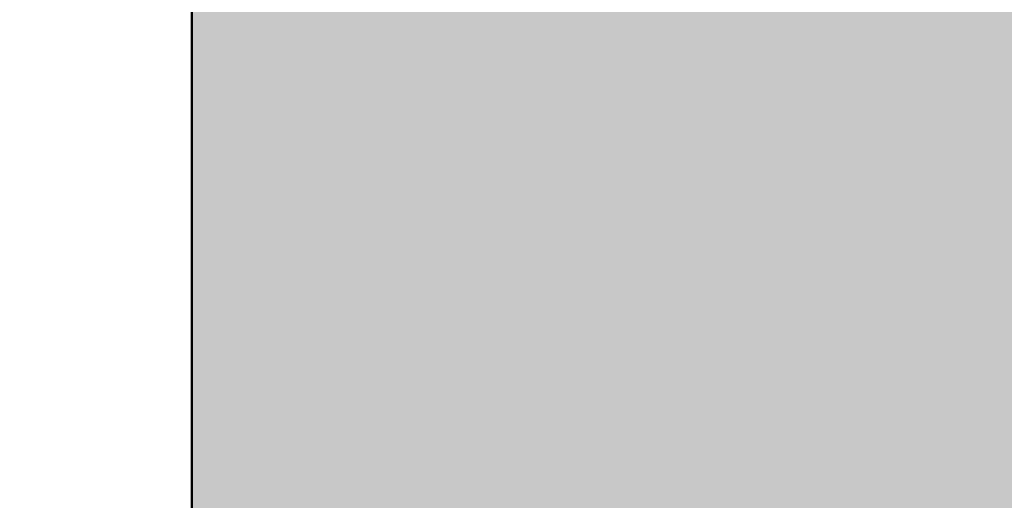
# Model space of a CAD drawing. Units: millimetres. Extents: x 0 to 2267, y 0 to 1823.
# Tile 29 of 256: x 1590 to 1611, y 1216 to 1226. Entities that reach past the tile are written whole.
import ezdxf

# ---------------------------------------------------------------- set-up
doc = ezdxf.new("R2010")
doc.units = ezdxf.units.MM
doc.header["$MEASUREMENT"] = 0
doc.layers.add('M-HATC', color=252, linetype='Continuous', lineweight=18)
doc.layers.add('M-OUTL', color=7, linetype='Continuous', lineweight=50)

msp = doc.modelspace()

# ---------------------------------------------------------------- hatches: boundary and pattern name
at = {"layer": 'M-HATC'}
h = msp.add_hatch(color=256, dxfattribs=at)
h.dxf.hatch_style = 1
h.paths.add_polyline_path([(2055.771, 1603.062), (1381.087, 1603.062), (1381.087, 1598.062), (2055.771, 1598.062)])
h.paths.add_polyline_path([(2055.771, 1598.062), (1381.087, 1598.062), (1381.087, 1593.062), (2055.771, 1593.062)])
h.paths.add_polyline_path([(2051.307, 1536.761), (1385.55, 1536.761), (1385.55, 1526.761), (1387.55, 1526.761), (1388.537, 1525.053), (1385.332, 1521.233), (1385.332, 1521.223), (2050.254, 1522.749), (2048.321, 1525.053), (2049.307, 1526.761), (2051.307, 1526.761)])
edge = h.paths.add_edge_path()
edge.add_arc((1847.535, 1379.149), 135, 222.60306, 222.89085, ccw=False)
edge.add_line((1748.166, 1287.766), (1683.092, 1287.766))
edge.add_arc((1583.724, 1379.149), 135, 317.10915, 317.39694, ccw=False)
edge.add_arc((1678.969, 1290.671), 5, 222.8909, 317.1091, ccw=False)
edge.add_arc((1774.213, 1379.149), 135, 222.60306, 222.89085, ccw=False)
edge.add_line((1674.845, 1287.766), (1609.771, 1287.766))
edge.add_arc((1510.403, 1379.149), 135, 317.10915, 317.39694, ccw=False)
edge.add_arc((1605.647, 1290.671), 5, 222.8909, 317.1091, ccw=False)
edge.add_arc((1700.892, 1379.149), 135, 222.60306, 222.89085, ccw=False)
edge.add_line((1601.524, 1287.766), (1536.45, 1287.766))
edge.add_arc((1437.081, 1379.149), 135, 317.10915, 317.39694, ccw=False)
edge.add_arc((1532.326, 1290.671), 5, 222.8909, 317.1091, ccw=False)
edge.add_arc((1627.571, 1379.149), 135, 222.60306, 222.89085, ccw=False)
edge.add_line((1528.203, 1287.766), (1505.929, 1287.766))
edge.add_spline(control_points=[(1505.929, 1287.766), (1504.262, 1287.766), (1504.262, 1282.766), (1505.929, 1282.766)], knot_values=[0, 0, 0, 0, 5, 5, 5, 5], degree=3, periodic=0)
edge.add_line((1505.929, 1282.766), (1930.929, 1282.766))
edge.add_spline(control_points=[(1930.929, 1282.766), (1932.596, 1282.766), (1932.596, 1287.766), (1930.929, 1287.766)], knot_values=[0, 0, 0, 0, 5, 5, 5, 5], degree=3, periodic=0)
edge.add_line((1930.929, 1287.766), (1903.056, 1287.766))
edge.add_arc((1803.688, 1379.149), 135, 317.10915, 317.39694, ccw=False)
edge.add_arc((1898.932, 1290.671), 5, 222.8909, 317.1091, ccw=False)
edge.add_arc((1994.177, 1379.149), 135, 222.60306, 222.89085, ccw=False)
edge.add_line((1894.809, 1287.766), (1829.735, 1287.766))
edge.add_arc((1730.366, 1379.149), 135, 317.10915, 317.39694, ccw=False)
edge.add_arc((1825.611, 1290.671), 5, 222.8909, 317.1091, ccw=False)
edge.add_arc((1920.856, 1379.149), 135, 222.60306, 222.89085, ccw=False)
edge.add_line((1821.487, 1287.766), (1756.413, 1287.766))
edge.add_arc((1657.045, 1379.149), 135, 317.10915, 317.39694, ccw=False)
edge.add_arc((1752.29, 1290.671), 5, 222.8909, 317.1091, ccw=False)
edge = h.paths.add_edge_path()
edge.add_spline(control_points=[(1843.429, 1227.247), (1845.096, 1227.247), (1845.096, 1232.247), (1843.429, 1232.247)], knot_values=[0, 0, 0, 0, 5, 5, 5, 5], degree=3, periodic=0)
edge.add_line((1843.429, 1232.247), (1593.429, 1232.247))
edge.add_spline(control_points=[(1593.429, 1232.247), (1591.762, 1232.247), (1591.762, 1227.247), (1593.429, 1227.247)], knot_values=[0, 0, 0, 0, 5, 5, 5, 5], degree=3, periodic=0)
edge.add_line((1593.429, 1227.247), (1843.429, 1227.247))
h.paths.add_polyline_path([(1905.929, 1127.417), (1530.929, 1127.417, 0.414214), (1520.929, 1117.417), (1530.929, 1117.417), (1915.929, 1117.417, 0.414214)])
edge = h.paths.add_edge_path()
edge.add_arc((1397.086, 1498.408), 12.73, 90.7821, 190.8787, ccw=False)
edge.add_line((1396.912, 1511.136), (1428.01, 1511.349))
edge.add_line((1428.01, 1511.349), (1433.01, 1511.349))
edge.add_line((1433.01, 1511.349), (1434.439, 1511.349))
edge.add_arc((1419.474, 1498.08), 20, 41.561, 74.0821)
edge.add_line((1424.959, 1517.314), (1399.935, 1517.256))
edge.add_spline(control_points=[(1399.931, 1517.256), (1399.884, 1517.213), (1399.833, 1517.169), (1399.777, 1517.124)], knot_values=[11.567499, 11.567499, 11.567499, 11.567499, 11.814249, 11.814249, 11.814249, 11.814249], degree=3, periodic=0)
edge.add_spline(control_points=[(1399.633, 1517.01), (1399.583, 1516.972), (1399.531, 1516.934), (1399.476, 1516.895)], knot_values=[11.167718, 11.167718, 11.167718, 11.167718, 11.365188, 11.365188, 11.365188, 11.365188], degree=3, periodic=0)
edge.add_spline(control_points=[(1399.34, 1516.8), (1399.151, 1516.672), (1398.938, 1516.538), (1398.704, 1516.399)], knot_values=[10.376405, 10.376405, 10.376405, 10.376405, 11.00994, 11.00994, 11.00994, 11.00994], degree=3, periodic=0)
edge.add_spline(control_points=[(1398.657, 1516.372), (1398.579, 1516.326), (1398.498, 1516.28), (1398.415, 1516.233)], knot_values=[10.125175, 10.125175, 10.125175, 10.125175, 10.334406, 10.334406, 10.334406, 10.334406], degree=3, periodic=0)
edge.add_spline(control_points=[(1398.264, 1516.149), (1398.196, 1516.111), (1398.126, 1516.073), (1398.055, 1516.035)], knot_values=[9.832246, 9.832246, 9.832246, 9.832246, 9.999658, 9.999658, 9.999658, 9.999658], degree=3, periodic=0)
edge.add_spline(control_points=[(1397.999, 1516.005), (1397.731, 1515.862), (1397.446, 1515.717), (1397.147, 1515.571)], knot_values=[9.161808, 9.161808, 9.161808, 9.161808, 9.787769, 9.787769, 9.787769, 9.787769], degree=3, periodic=0)
edge.add_spline(control_points=[(1397.147, 1515.571), (1396.842, 1515.423), (1396.522, 1515.274), (1396.191, 1515.126)], knot_values=[8.524455, 8.524455, 8.524455, 8.524455, 9.161808, 9.161808, 9.161808, 9.161808], degree=3, periodic=0)
edge.add_spline(control_points=[(1396.078, 1515.076), (1395.985, 1515.035), (1395.892, 1514.994), (1395.798, 1514.953)], knot_values=[8.275193, 8.275193, 8.275193, 8.275193, 8.451726, 8.451726, 8.451726, 8.451726], degree=3, periodic=0)
edge.add_spline(control_points=[(1395.602, 1514.869), (1395.5, 1514.826), (1395.397, 1514.782), (1395.293, 1514.739)], knot_values=[7.962917, 7.962917, 7.962917, 7.962917, 8.152764, 8.152764, 8.152764, 8.152764], degree=3, periodic=0)
edge.add_spline(control_points=[(1395.212, 1514.706), (1394.828, 1514.547), (1394.435, 1514.393), (1394.036, 1514.244)], knot_values=[7.21254, 7.21254, 7.21254, 7.21254, 7.913148, 7.913148, 7.913148, 7.913148], degree=3, periodic=0)
edge.add_spline(control_points=[(1394.036, 1514.244), (1393.708, 1514.121), (1393.375, 1514.003), (1393.043, 1513.889)], knot_values=[6.633733, 6.633733, 6.633733, 6.633733, 7.21254, 7.21254, 7.21254, 7.21254], degree=3, periodic=0)
edge.add_spline(control_points=[(1392.821, 1513.815), (1392.72, 1513.781), (1392.618, 1513.748), (1392.517, 1513.715)], knot_values=[6.328796, 6.328796, 6.328796, 6.328796, 6.505493, 6.505493, 6.505493, 6.505493], degree=3, periodic=0)
edge.add_spline(control_points=[(1392.517, 1513.715), (1392.319, 1513.652), (1392.121, 1513.59), (1391.924, 1513.531)], knot_values=[5.984605, 5.984605, 5.984605, 5.984605, 6.328796, 6.328796, 6.328796, 6.328796], degree=3, periodic=0)
edge.add_spline(control_points=[(1391.792, 1513.491), (1391.312, 1513.35), (1390.838, 1513.224), (1390.378, 1513.117)], knot_values=[5.066697, 5.066697, 5.066697, 5.066697, 5.907055, 5.907055, 5.907055, 5.907055], degree=3, periodic=0)
edge.add_spline(control_points=[(1390.378, 1513.117), (1390.18, 1513.071), (1389.984, 1513.028), (1389.791, 1512.99)], knot_values=[4.70367, 4.70367, 4.70367, 4.70367, 5.066695, 5.066695, 5.066695, 5.066695], degree=3, periodic=0)
edge.add_spline(control_points=[(1389.422, 1512.92), (1389.246, 1512.889), (1389.073, 1512.862), (1388.904, 1512.838)], knot_values=[4.130571, 4.130571, 4.130571, 4.130571, 4.469816, 4.469816, 4.469816, 4.469816], degree=3, periodic=0)
edge.add_spline(control_points=[(1388.904, 1512.838), (1388.591, 1512.795), (1388.291, 1512.764), (1388.007, 1512.749)], knot_values=[3.504031, 3.504031, 3.504031, 3.504031, 4.130571, 4.130571, 4.130571, 4.130571], degree=3, periodic=0)
edge.add_spline(control_points=[(1387.936, 1512.746), (1387.854, 1512.742), (1387.773, 1512.74), (1387.694, 1512.739)], knot_values=[3.268866, 3.268866, 3.268866, 3.268866, 3.451164, 3.451164, 3.451164, 3.451164], degree=3, periodic=0)
edge.add_spline(control_points=[(1387.335, 1512.744), (1387.208, 1512.75), (1387.085, 1512.76), (1386.967, 1512.774)], knot_values=[2.670686, 2.670686, 2.670686, 2.670686, 2.984, 2.984, 2.984, 2.984], degree=3, periodic=0)
edge.add_spline(control_points=[(1386.833, 1512.792), (1386.821, 1512.794), (1386.809, 1512.796), (1386.797, 1512.798)], knot_values=[2.516981, 2.516981, 2.516981, 2.516981, 2.549528, 2.549528, 2.549528, 2.549528], degree=3, periodic=0)
edge.add_spline(control_points=[(1386.453, 1512.873), (1386.426, 1512.881), (1386.399, 1512.889), (1386.373, 1512.897)], knot_values=[2.095869, 2.095869, 2.095869, 2.095869, 2.17941, 2.17941, 2.17941, 2.17941], degree=3, periodic=0)
edge.add_spline(control_points=[(1386.069, 1513.019), (1386.063, 1513.022), (1386.058, 1513.025), (1386.052, 1513.028)], knot_values=[1.72453, 1.72453, 1.72453, 1.72453, 1.745933, 1.745933, 1.745933, 1.745933], degree=3, periodic=0)
edge.add_arc((1399.474, 1498.08), 20, 131.8243, 180)
edge.add_arc((1630.334, 1505.548), 250.971, 181.70518, 236.42798)
edge.add_arc((1605.34, 1483.304), 218.782, 238.66083, 243.34961)
edge.add_arc((1647.091, 1510.359), 262.899, 183.12984, 237.85344, ccw=False)
h.paths.add_polyline_path([(1406.537, 1391.964, 0.149382), (1491.551, 1296.442, -0.129517)], flags=17)
edge = h.paths.add_edge_path()
edge.add_arc((2037.384, 1498.08), 20, 0, 48.2659)
edge.add_spline(control_points=[(2050.697, 1513.005), (2050.651, 1512.985), (2050.603, 1512.966), (2050.554, 1512.948)], knot_values=[1.835652, 1.835652, 1.835652, 1.835652, 2.000781, 2.000781, 2.000781, 2.000781], degree=3, periodic=0)
edge.add_spline(control_points=[(2050.462, 1512.917), (2050.479, 1512.922), (2050.496, 1512.928), (2050.513, 1512.934)], knot_values=[2.045477, 2.045477, 2.045477, 2.045477, 2.101389, 2.101389, 2.101389, 2.101389], degree=3, periodic=0)
edge.add_spline(control_points=[(2050.129, 1512.834), (2050.198, 1512.847), (2050.266, 1512.862), (2050.331, 1512.879)], knot_values=[2.237629, 2.237629, 2.237629, 2.237629, 2.435841, 2.435841, 2.435841, 2.435841], degree=3, periodic=0)
edge.add_spline(control_points=[(2050.095, 1512.828), (2050.106, 1512.83), (2050.118, 1512.832), (2050.129, 1512.834)], knot_values=[2.435841, 2.435841, 2.435841, 2.435841, 2.468321, 2.468321, 2.468321, 2.468321], degree=3, periodic=0)
edge.add_spline(control_points=[(2049.784, 1512.785), (2049.855, 1512.792), (2049.924, 1512.801), (2049.992, 1512.811)], knot_values=[2.563852, 2.563852, 2.563852, 2.563852, 2.748541, 2.748541, 2.748541, 2.748541], degree=3, periodic=0)
edge.add_spline(control_points=[(2049.405, 1512.762), (2049.536, 1512.765), (2049.663, 1512.773), (2049.784, 1512.785)], knot_values=[2.748541, 2.748541, 2.748541, 2.748541, 3.064882, 3.064882, 3.064882, 3.064882], degree=3, periodic=0)
edge.add_spline(control_points=[(2049.17, 1512.76), (2049.234, 1512.759), (2049.297, 1512.759), (2049.358, 1512.761)], knot_values=[3.102309, 3.102309, 3.102309, 3.102309, 3.2503, 3.2503, 3.2503, 3.2503], degree=3, periodic=0)
edge.add_spline(control_points=[(2048.857, 1512.769), (2048.964, 1512.764), (2049.068, 1512.761), (2049.17, 1512.76)], knot_values=[3.2503, 3.2503, 3.2503, 3.2503, 3.486069, 3.486069, 3.486069, 3.486069], degree=3, periodic=0)
edge.add_spline(control_points=[(2048.692, 1512.779), (2048.373, 1512.801), (2048.035, 1512.841), (2047.682, 1512.897)], knot_values=[3.606429, 3.606429, 3.606429, 3.606429, 4.2989, 4.2989, 4.2989, 4.2989], degree=3, periodic=0)
edge.add_spline(control_points=[(2047.682, 1512.897), (2047.546, 1512.919), (2047.408, 1512.942), (2047.268, 1512.969)], knot_values=[4.2989, 4.2989, 4.2989, 4.2989, 4.565769, 4.565769, 4.565769, 4.565769], degree=3, periodic=0)
edge.add_spline(control_points=[(2047.268, 1512.969), (2047.145, 1512.991), (2047.021, 1513.016), (2046.895, 1513.042)], knot_values=[4.565769, 4.565769, 4.565769, 4.565769, 4.799971, 4.799971, 4.799971, 4.799971], degree=3, periodic=0)
edge.add_spline(control_points=[(2046.895, 1513.042), (2046.529, 1513.119), (2046.151, 1513.209), (2045.768, 1513.311)], knot_values=[4.799971, 4.799971, 4.799971, 4.799971, 5.483718, 5.483718, 5.483718, 5.483718], degree=3, periodic=0)
edge.add_spline(control_points=[(2045.768, 1513.311), (2045.372, 1513.415), (2044.97, 1513.532), (2044.566, 1513.659)], knot_values=[5.483718, 5.483718, 5.483718, 5.483718, 6.187866, 6.187866, 6.187866, 6.187866], degree=3, periodic=0)
edge.add_spline(control_points=[(2044.566, 1513.659), (2044.415, 1513.706), (2044.263, 1513.755), (2044.112, 1513.805)], knot_values=[6.187866, 6.187866, 6.187866, 6.187866, 6.451551, 6.451551, 6.451551, 6.451551], degree=3, periodic=0)
edge.add_spline(control_points=[(2044.112, 1513.805), (2043.997, 1513.843), (2043.882, 1513.881), (2043.767, 1513.92)], knot_values=[6.451551, 6.451551, 6.451551, 6.451551, 6.651434, 6.651434, 6.651434, 6.651434], degree=3, periodic=0)
edge.add_spline(control_points=[(2043.767, 1513.92), (2043.372, 1514.055), (2042.977, 1514.198), (2042.589, 1514.346)], knot_values=[6.651434, 6.651434, 6.651434, 6.651434, 7.338879, 7.338879, 7.338879, 7.338879], degree=3, periodic=0)
edge.add_spline(control_points=[(2042.589, 1514.346), (2042.164, 1514.507), (2041.746, 1514.675), (2041.341, 1514.846)], knot_values=[7.338879, 7.338879, 7.338879, 7.338879, 8.089209, 8.089209, 8.089209, 8.089209], degree=3, periodic=0)
edge.add_spline(control_points=[(2041.341, 1514.846), (2041.103, 1514.946), (2040.869, 1515.048), (2040.64, 1515.15)], knot_values=[8.089209, 8.089209, 8.089209, 8.089209, 8.529587, 8.529587, 8.529587, 8.529587], degree=3, periodic=0)
edge.add_spline(control_points=[(2040.51, 1515.209), (2040.082, 1515.402), (2039.675, 1515.597), (2039.295, 1515.789)], knot_values=[8.613818, 8.613818, 8.613818, 8.613818, 9.44571, 9.44571, 9.44571, 9.44571], degree=3, periodic=0)
edge.add_spline(control_points=[(2039.295, 1515.789), (2039.062, 1515.907), (2038.839, 1516.025), (2038.629, 1516.14)], knot_values=[9.44571, 9.44571, 9.44571, 9.44571, 9.956404, 9.956404, 9.956404, 9.956404], degree=3, periodic=0)
edge.add_spline(control_points=[(2038.629, 1516.14), (2038.519, 1516.2), (2038.412, 1516.26), (2038.309, 1516.319)], knot_values=[9.956404, 9.956404, 9.956404, 9.956404, 10.223542, 10.223542, 10.223542, 10.223542], degree=3, periodic=0)
edge.add_spline(control_points=[(2038.309, 1516.319), (2038.214, 1516.374), (2038.122, 1516.428), (2038.033, 1516.481)], knot_values=[10.223542, 10.223542, 10.223542, 10.223542, 10.47051, 10.47051, 10.47051, 10.47051], degree=3, periodic=0)
edge.add_spline(control_points=[(2038.033, 1516.481), (2037.786, 1516.63), (2037.564, 1516.773), (2037.372, 1516.909)], knot_values=[10.47051, 10.47051, 10.47051, 10.47051, 11.15767, 11.15767, 11.15767, 11.15767], degree=3, periodic=0)
edge.add_spline(control_points=[(2037.372, 1516.909), (2037.279, 1516.975), (2037.193, 1517.04), (2037.114, 1517.102)], knot_values=[11.15767, 11.15767, 11.15767, 11.15767, 11.49227, 11.49227, 11.49227, 11.49227], degree=3, periodic=0)
edge.add_spline(control_points=[(2036.856, 1517.326), (2036.915, 1517.269), (2036.981, 1517.21), (2037.056, 1517.149)], knot_values=[11.577341, 11.577341, 11.577341, 11.577341, 11.91035, 11.91035, 11.91035, 11.91035], degree=3, periodic=0)
edge.add_spline(control_points=[(2036.807, 1517.375), (2036.823, 1517.359), (2036.839, 1517.342), (2036.856, 1517.326)], knot_values=[11.91035, 11.91035, 11.91035, 11.91035, 12.007402, 12.007402, 12.007402, 12.007402], degree=3, periodic=0)
edge.add_spline(control_points=[(2036.702, 1517.494), (2036.71, 1517.483), (2036.72, 1517.472), (2036.729, 1517.461)], knot_values=[12.184155, 12.184155, 12.184155, 12.184155, 12.255409, 12.255409, 12.255409, 12.255409], degree=3, periodic=0)
edge.add_spline(control_points=[(2036.616, 1517.621), (2036.62, 1517.613), (2036.624, 1517.606), (2036.629, 1517.598)], knot_values=[12.487913, 12.487913, 12.487913, 12.487913, 12.541035, 12.541035, 12.541035, 12.541035], degree=3, periodic=0)
edge.add_spline(control_points=[(2036.563, 1517.786), (2036.564, 1517.779), (2036.564, 1517.773), (2036.565, 1517.766)], knot_values=[12.911761, 12.911761, 12.911761, 12.911761, 12.968286, 12.968286, 12.968286, 12.968286], degree=3, periodic=0)
edge.add_spline(control_points=[(2036.617, 1517.93), (2036.612, 1517.926), (2036.609, 1517.921), (2036.605, 1517.916)], knot_values=[13.382527, 13.382527, 13.382527, 13.382527, 13.433791, 13.433791, 13.433791, 13.433791], degree=3, periodic=0)
edge.add_spline(control_points=[(2036.749, 1518.017), (2036.736, 1518.012), (2036.724, 1518.006), (2036.712, 1518)], knot_values=[13.726299, 13.726299, 13.726299, 13.726299, 13.809928, 13.809928, 13.809928, 13.809928], degree=3, periodic=0)
edge.add_spline(control_points=[(2036.86, 1518.053), (2036.839, 1518.047), (2036.818, 1518.042), (2036.799, 1518.035)], knot_values=[13.910887, 13.910887, 13.910887, 13.910887, 14.02153, 14.02153, 14.02153, 14.02153], degree=3, periodic=0)
edge.add_line((2036.964, 1518.08), (2032.384, 1518.08))
edge.add_line((2032.384, 1518.08), (2027.384, 1518.08))
edge.add_line((2027.384, 1518.08), (2022.384, 1518.08))
edge.add_line((2022.384, 1518.08), (2017.384, 1518.08))
edge.add_arc((2017.384, 1498.08), 20, 90, 138.439)
edge.add_line((2002.419, 1511.349), (2003.848, 1511.349))
edge.add_line((2003.848, 1511.349), (2008.848, 1511.349))
edge.add_line((2008.848, 1511.349), (2039.772, 1511.138))
edge.add_arc((2039.772, 1498.408), 12.73, -10.8787, 90, ccw=False)
edge.add_arc((1789.767, 1510.359), 262.899, 302.14656, 356.87016, ccw=False)
edge.add_arc((1831.518, 1483.304), 218.782, 296.65039, 301.33917)
edge.add_arc((1806.524, 1505.548), 250.971, 303.57202, 358.29482)
h.paths.add_polyline_path([(2030.321, 1391.964, -0.129517), (1945.307, 1296.442, 0.149382)], flags=17)
edge = h.paths.add_edge_path()
edge.add_spline(control_points=[(2037.246, 1518.082), (2037.29, 1518.081), (2037.336, 1518.08), (2037.384, 1518.08)], knot_values=[0.000012, 0.000012, 0.000012, 0.000012, 0.144754, 0.144754, 0.144754, 0.144754], degree=3, periodic=0)
edge.add_line((2037.336, 1518.08), (2037.01, 1518.08))
edge.add_spline(control_points=[(2037.01, 1518.08), (2036.982, 1518.077), (2036.956, 1518.073), (2036.931, 1518.068)], knot_values=[14.13465, 14.13465, 14.13465, 14.13465, 14.247197, 14.247197, 14.247197, 14.247197], degree=3, periodic=0)
edge.add_spline(control_points=[(2036.931, 1518.068), (2036.928, 1518.067), (2036.924, 1518.067), (2036.921, 1518.066)], knot_values=[14.118315, 14.118315, 14.118315, 14.118315, 14.13465, 14.13465, 14.13465, 14.13465], degree=3, periodic=0)
edge.add_spline(control_points=[(2036.921, 1518.066), (2036.912, 1518.064), (2036.903, 1518.063), (2036.895, 1518.061)], knot_values=[14.078086, 14.078086, 14.078086, 14.078086, 14.118315, 14.118315, 14.118315, 14.118315], degree=3, periodic=0)
edge.add_spline(control_points=[(2036.895, 1518.061), (2036.883, 1518.058), (2036.872, 1518.056), (2036.86, 1518.053)], knot_values=[14.02153, 14.02153, 14.02153, 14.02153, 14.078086, 14.078086, 14.078086, 14.078086], degree=3, periodic=0)
edge.add_spline(control_points=[(2036.86, 1518.053), (2036.839, 1518.047), (2036.818, 1518.042), (2036.799, 1518.035)], knot_values=[13.910887, 13.910887, 13.910887, 13.910887, 14.02153, 14.02153, 14.02153, 14.02153], degree=3, periodic=0)
edge.add_spline(control_points=[(2036.799, 1518.035), (2036.798, 1518.035), (2036.797, 1518.035), (2036.797, 1518.035)], knot_values=[13.906906, 13.906906, 13.906906, 13.906906, 13.910887, 13.910887, 13.910887, 13.910887], degree=3, periodic=0)
edge.add_spline(control_points=[(2036.797, 1518.035), (2036.788, 1518.032), (2036.78, 1518.029), (2036.772, 1518.026)], knot_values=[13.857826, 13.857826, 13.857826, 13.857826, 13.906906, 13.906906, 13.906906, 13.906906], degree=3, periodic=0)
edge.add_spline(control_points=[(2036.772, 1518.026), (2036.764, 1518.023), (2036.756, 1518.02), (2036.749, 1518.017)], knot_values=[13.809928, 13.809928, 13.809928, 13.809928, 13.857826, 13.857826, 13.857826, 13.857826], degree=3, periodic=0)
edge.add_spline(control_points=[(2036.749, 1518.017), (2036.736, 1518.012), (2036.724, 1518.006), (2036.712, 1518)], knot_values=[13.726299, 13.726299, 13.726299, 13.726299, 13.809928, 13.809928, 13.809928, 13.809928], degree=3, periodic=0)
edge.add_spline(control_points=[(2036.712, 1518), (2036.712, 1518), (2036.712, 1518), (2036.711, 1518)], knot_values=[13.723993, 13.723993, 13.723993, 13.723993, 13.726299, 13.726299, 13.726299, 13.726299], degree=3, periodic=0)
edge.add_spline(control_points=[(2036.711, 1518), (2036.706, 1517.997), (2036.701, 1517.994), (2036.696, 1517.992)], knot_values=[13.686536, 13.686536, 13.686536, 13.686536, 13.723993, 13.723993, 13.723993, 13.723993], degree=3, periodic=0)
edge.add_spline(control_points=[(2036.696, 1517.992), (2036.692, 1517.989), (2036.687, 1517.987), (2036.683, 1517.984)], knot_values=[13.651251, 13.651251, 13.651251, 13.651251, 13.686536, 13.686536, 13.686536, 13.686536], degree=3, periodic=0)
edge.add_spline(control_points=[(2036.683, 1517.984), (2036.676, 1517.98), (2036.67, 1517.976), (2036.664, 1517.971)], knot_values=[13.596804, 13.596804, 13.596804, 13.596804, 13.651251, 13.651251, 13.651251, 13.651251], degree=3, periodic=0)
edge.add_spline(control_points=[(2036.664, 1517.971), (2036.664, 1517.971), (2036.663, 1517.971), (2036.663, 1517.971)], knot_values=[13.593956, 13.593956, 13.593956, 13.593956, 13.596804, 13.596804, 13.596804, 13.596804], degree=3, periodic=0)
edge.add_spline(control_points=[(2036.663, 1517.971), (2036.66, 1517.969), (2036.658, 1517.967), (2036.655, 1517.965)], knot_values=[13.570322, 13.570322, 13.570322, 13.570322, 13.593956, 13.593956, 13.593956, 13.593956], degree=3, periodic=0)
edge.add_spline(control_points=[(2036.655, 1517.965), (2036.653, 1517.963), (2036.65, 1517.961), (2036.647, 1517.959)], knot_values=[13.545477, 13.545477, 13.545477, 13.545477, 13.570322, 13.570322, 13.570322, 13.570322], degree=3, periodic=0)
edge.add_spline(control_points=[(2036.647, 1517.959), (2036.647, 1517.959), (2036.647, 1517.959), (2036.647, 1517.959)], knot_values=[13.543931, 13.543931, 13.543931, 13.543931, 13.545477, 13.545477, 13.545477, 13.545477], degree=3, periodic=0)
edge.add_spline(control_points=[(2036.647, 1517.959), (2036.641, 1517.954), (2036.636, 1517.949), (2036.631, 1517.945)], knot_values=[13.488237, 13.488237, 13.488237, 13.488237, 13.543931, 13.543931, 13.543931, 13.543931], degree=3, periodic=0)
edge.add_spline(control_points=[(2036.631, 1517.945), (2036.628, 1517.942), (2036.626, 1517.94), (2036.623, 1517.937)], knot_values=[13.460307, 13.460307, 13.460307, 13.460307, 13.488237, 13.488237, 13.488237, 13.488237], degree=3, periodic=0)
edge.add_spline(control_points=[(2036.623, 1517.937), (2036.622, 1517.936), (2036.62, 1517.934), (2036.618, 1517.932)], knot_values=[13.439712, 13.439712, 13.439712, 13.439712, 13.460307, 13.460307, 13.460307, 13.460307], degree=3, periodic=0)
edge.add_spline(control_points=[(2036.618, 1517.932), (2036.618, 1517.931), (2036.617, 1517.931), (2036.617, 1517.93)], knot_values=[13.433791, 13.433791, 13.433791, 13.433791, 13.439712, 13.439712, 13.439712, 13.439712], degree=3, periodic=0)
edge.add_spline(control_points=[(2036.617, 1517.93), (2036.612, 1517.926), (2036.609, 1517.921), (2036.605, 1517.916)], knot_values=[13.382527, 13.382527, 13.382527, 13.382527, 13.433791, 13.433791, 13.433791, 13.433791], degree=3, periodic=0)
edge.add_spline(control_points=[(2036.605, 1517.916), (2036.603, 1517.913), (2036.6, 1517.91), (2036.598, 1517.907)], knot_values=[13.350017, 13.350017, 13.350017, 13.350017, 13.382527, 13.382527, 13.382527, 13.382527], degree=3, periodic=0)
edge.add_spline(control_points=[(2036.598, 1517.907), (2036.597, 1517.906), (2036.596, 1517.904), (2036.595, 1517.903)], knot_values=[13.333922, 13.333922, 13.333922, 13.333922, 13.350017, 13.350017, 13.350017, 13.350017], degree=3, periodic=0)
edge.add_spline(control_points=[(2036.595, 1517.903), (2036.595, 1517.902), (2036.594, 1517.901), (2036.593, 1517.9)], knot_values=[13.323828, 13.323828, 13.323828, 13.323828, 13.333922, 13.333922, 13.333922, 13.333922], degree=3, periodic=0)
edge.add_spline(control_points=[(2036.593, 1517.9), (2036.59, 1517.895), (2036.588, 1517.891), (2036.585, 1517.886)], knot_values=[13.277545, 13.277545, 13.277545, 13.277545, 13.323828, 13.323828, 13.323828, 13.323828], degree=3, periodic=0)
edge.add_spline(control_points=[(2036.585, 1517.886), (2036.584, 1517.883), (2036.582, 1517.879), (2036.58, 1517.875)], knot_values=[13.240119, 13.240119, 13.240119, 13.240119, 13.277545, 13.277545, 13.277545, 13.277545], degree=3, periodic=0)
edge.add_spline(control_points=[(2036.58, 1517.875), (2036.58, 1517.874), (2036.579, 1517.873), (2036.578, 1517.872)], knot_values=[13.228211, 13.228211, 13.228211, 13.228211, 13.240119, 13.240119, 13.240119, 13.240119], degree=3, periodic=0)
edge.add_spline(control_points=[(2036.578, 1517.872), (2036.578, 1517.87), (2036.577, 1517.869), (2036.577, 1517.868)], knot_values=[13.215717, 13.215717, 13.215717, 13.215717, 13.228211, 13.228211, 13.228211, 13.228211], degree=3, periodic=0)
edge.add_spline(control_points=[(2036.577, 1517.868), (2036.575, 1517.864), (2036.574, 1517.86), (2036.573, 1517.857)], knot_values=[13.179847, 13.179847, 13.179847, 13.179847, 13.215717, 13.215717, 13.215717, 13.215717], degree=3, periodic=0)
edge.add_spline(control_points=[(2036.573, 1517.857), (2036.571, 1517.851), (2036.57, 1517.846), (2036.569, 1517.841)], knot_values=[13.132017, 13.132017, 13.132017, 13.132017, 13.179847, 13.179847, 13.179847, 13.179847], degree=3, periodic=0)
edge.add_spline(control_points=[(2036.569, 1517.841), (2036.568, 1517.84), (2036.568, 1517.839), (2036.568, 1517.838)], knot_values=[13.122482, 13.122482, 13.122482, 13.122482, 13.132017, 13.132017, 13.132017, 13.132017], degree=3, periodic=0)
edge.add_spline(control_points=[(2036.568, 1517.838), (2036.568, 1517.836), (2036.567, 1517.835), (2036.567, 1517.833)], knot_values=[13.105592, 13.105592, 13.105592, 13.105592, 13.122482, 13.122482, 13.122482, 13.122482], degree=3, periodic=0)
edge.add_spline(control_points=[(2036.567, 1517.833), (2036.566, 1517.829), (2036.566, 1517.826), (2036.565, 1517.822)], knot_values=[13.074063, 13.074063, 13.074063, 13.074063, 13.105592, 13.105592, 13.105592, 13.105592], degree=3, periodic=0)
edge.add_spline(control_points=[(2036.565, 1517.822), (2036.565, 1517.822), (2036.565, 1517.822), (2036.565, 1517.822)], knot_values=[13.074043, 13.074043, 13.074043, 13.074043, 13.074063, 13.074063, 13.074063, 13.074063], degree=3, periodic=0)
edge.add_spline(control_points=[(2036.565, 1517.822), (2036.564, 1517.816), (2036.564, 1517.811), (2036.564, 1517.805)], knot_values=[13.021884, 13.021884, 13.021884, 13.021884, 13.074043, 13.074043, 13.074043, 13.074043], degree=3, periodic=0)
edge.add_spline(control_points=[(2036.564, 1517.805), (2036.564, 1517.804), (2036.564, 1517.803), (2036.564, 1517.803)], knot_values=[13.01674, 13.01674, 13.01674, 13.01674, 13.021884, 13.021884, 13.021884, 13.021884], degree=3, periodic=0)
edge.add_spline(control_points=[(2036.564, 1517.803), (2036.563, 1517.801), (2036.563, 1517.798), (2036.563, 1517.796)], knot_values=[12.996438, 12.996438, 12.996438, 12.996438, 13.01674, 13.01674, 13.01674, 13.01674], degree=3, periodic=0)
edge.add_spline(control_points=[(2036.563, 1517.796), (2036.563, 1517.793), (2036.563, 1517.789), (2036.563, 1517.786)], knot_values=[12.968286, 12.968286, 12.968286, 12.968286, 12.996438, 12.996438, 12.996438, 12.996438], degree=3, periodic=0)
edge.add_spline(control_points=[(2036.563, 1517.786), (2036.564, 1517.779), (2036.564, 1517.773), (2036.565, 1517.766)], knot_values=[12.911761, 12.911761, 12.911761, 12.911761, 12.968286, 12.968286, 12.968286, 12.968286], degree=3, periodic=0)
edge.add_spline(control_points=[(2036.565, 1517.766), (2036.565, 1517.766), (2036.565, 1517.766), (2036.565, 1517.766)], knot_values=[12.911017, 12.911017, 12.911017, 12.911017, 12.911761, 12.911761, 12.911761, 12.911761], degree=3, periodic=0)
edge.add_spline(control_points=[(2036.565, 1517.766), (2036.565, 1517.762), (2036.566, 1517.759), (2036.566, 1517.756)], knot_values=[12.88528, 12.88528, 12.88528, 12.88528, 12.911017, 12.911017, 12.911017, 12.911017], degree=3, periodic=0)
edge.add_spline(control_points=[(2036.566, 1517.756), (2036.567, 1517.753), (2036.567, 1517.751), (2036.568, 1517.748)], knot_values=[12.862519, 12.862519, 12.862519, 12.862519, 12.88528, 12.88528, 12.88528, 12.88528], degree=3, periodic=0)
edge.add_spline(control_points=[(2036.568, 1517.748), (2036.568, 1517.747), (2036.568, 1517.747), (2036.568, 1517.746)], knot_values=[12.858885, 12.858885, 12.858885, 12.858885, 12.862519, 12.862519, 12.862519, 12.862519], degree=3, periodic=0)
edge.add_spline(control_points=[(2036.568, 1517.746), (2036.569, 1517.74), (2036.571, 1517.733), (2036.572, 1517.726)], knot_values=[12.8053, 12.8053, 12.8053, 12.8053, 12.858885, 12.858885, 12.858885, 12.858885], degree=3, periodic=0)
edge.add_spline(control_points=[(2036.572, 1517.726), (2036.573, 1517.723), (2036.574, 1517.719), (2036.576, 1517.715)], knot_values=[12.775176, 12.775176, 12.775176, 12.775176, 12.8053, 12.8053, 12.8053, 12.8053], degree=3, periodic=0)
edge.add_spline(control_points=[(2036.576, 1517.715), (2036.576, 1517.713), (2036.577, 1517.71), (2036.578, 1517.708)], knot_values=[12.756759, 12.756759, 12.756759, 12.756759, 12.775176, 12.775176, 12.775176, 12.775176], degree=3, periodic=0)
edge.add_spline(control_points=[(2036.578, 1517.708), (2036.578, 1517.707), (2036.578, 1517.706), (2036.579, 1517.705)], knot_values=[12.748742, 12.748742, 12.748742, 12.748742, 12.756759, 12.756759, 12.756759, 12.756759], degree=3, periodic=0)
edge.add_spline(control_points=[(2036.579, 1517.705), (2036.581, 1517.698), (2036.583, 1517.692), (2036.586, 1517.685)], knot_values=[12.69959, 12.69959, 12.69959, 12.69959, 12.748742, 12.748742, 12.748742, 12.748742], degree=3, periodic=0)
edge.add_spline(control_points=[(2036.586, 1517.685), (2036.588, 1517.68), (2036.59, 1517.675), (2036.592, 1517.669)], knot_values=[12.659038, 12.659038, 12.659038, 12.659038, 12.69959, 12.69959, 12.69959, 12.69959], degree=3, periodic=0)
edge.add_spline(control_points=[(2036.592, 1517.669), (2036.594, 1517.665), (2036.596, 1517.66), (2036.598, 1517.656)], knot_values=[12.626806, 12.626806, 12.626806, 12.626806, 12.659038, 12.659038, 12.659038, 12.659038], degree=3, periodic=0)
edge.add_spline(control_points=[(2036.598, 1517.656), (2036.598, 1517.655), (2036.599, 1517.654), (2036.599, 1517.653)], knot_values=[12.619394, 12.619394, 12.619394, 12.619394, 12.626806, 12.626806, 12.626806, 12.626806], degree=3, periodic=0)
edge.add_spline(control_points=[(2036.599, 1517.653), (2036.604, 1517.642), (2036.61, 1517.632), (2036.616, 1517.621)], knot_values=[12.541039, 12.541039, 12.541039, 12.541039, 12.619394, 12.619394, 12.619394, 12.619394], degree=3, periodic=0)
edge.add_spline(control_points=[(2036.616, 1517.621), (2036.616, 1517.621), (2036.616, 1517.621), (2036.616, 1517.621)], knot_values=[12.541035, 12.541035, 12.541035, 12.541035, 12.541039, 12.541039, 12.541039, 12.541039], degree=3, periodic=0)
edge.add_spline(control_points=[(2036.616, 1517.621), (2036.62, 1517.613), (2036.624, 1517.606), (2036.629, 1517.598)], knot_values=[12.487913, 12.487913, 12.487913, 12.487913, 12.541035, 12.541035, 12.541035, 12.541035], degree=3, periodic=0)
edge.add_spline(control_points=[(2036.629, 1517.598), (2036.633, 1517.592), (2036.637, 1517.585), (2036.641, 1517.579)], knot_values=[12.443982, 12.443982, 12.443982, 12.443982, 12.487913, 12.487913, 12.487913, 12.487913], degree=3, periodic=0)
edge.add_spline(control_points=[(2036.641, 1517.579), (2036.641, 1517.578), (2036.642, 1517.576), (2036.643, 1517.575)], knot_values=[12.434996, 12.434996, 12.434996, 12.434996, 12.443982, 12.443982, 12.443982, 12.443982], degree=3, periodic=0)
edge.add_spline(control_points=[(2036.643, 1517.575), (2036.653, 1517.56), (2036.664, 1517.544), (2036.676, 1517.528)], knot_values=[12.329647, 12.329647, 12.329647, 12.329647, 12.434996, 12.434996, 12.434996, 12.434996], degree=3, periodic=0)
edge.add_spline(control_points=[(2036.676, 1517.528), (2036.684, 1517.517), (2036.693, 1517.505), (2036.702, 1517.494)], knot_values=[12.255409, 12.255409, 12.255409, 12.255409, 12.329647, 12.329647, 12.329647, 12.329647], degree=3, periodic=0)
edge.add_spline(control_points=[(2036.702, 1517.494), (2036.71, 1517.483), (2036.72, 1517.472), (2036.729, 1517.461)], knot_values=[12.184155, 12.184155, 12.184155, 12.184155, 12.255409, 12.255409, 12.255409, 12.255409], degree=3, periodic=0)
edge.add_spline(control_points=[(2036.729, 1517.461), (2036.744, 1517.444), (2036.759, 1517.426), (2036.775, 1517.409)], knot_values=[12.075961, 12.075961, 12.075961, 12.075961, 12.184155, 12.184155, 12.184155, 12.184155], degree=3, periodic=0)
edge.add_spline(control_points=[(2036.775, 1517.409), (2036.776, 1517.407), (2036.777, 1517.406), (2036.778, 1517.405)], knot_values=[12.069502, 12.069502, 12.069502, 12.069502, 12.075961, 12.075961, 12.075961, 12.075961], degree=3, periodic=0)
edge.add_spline(control_points=[(2036.778, 1517.405), (2036.788, 1517.395), (2036.797, 1517.385), (2036.807, 1517.375)], knot_values=[12.007402, 12.007402, 12.007402, 12.007402, 12.069502, 12.069502, 12.069502, 12.069502], degree=3, periodic=0)
edge.add_spline(control_points=[(2036.807, 1517.375), (2036.823, 1517.359), (2036.839, 1517.342), (2036.856, 1517.326)], knot_values=[11.91035, 11.91035, 11.91035, 11.91035, 12.007402, 12.007402, 12.007402, 12.007402], degree=3, periodic=0)
edge.add_spline(control_points=[(2036.856, 1517.326), (2036.915, 1517.269), (2036.981, 1517.21), (2037.056, 1517.149)], knot_values=[11.577341, 11.577341, 11.577341, 11.577341, 11.91035, 11.91035, 11.91035, 11.91035], degree=3, periodic=0)
edge.add_spline(control_points=[(2037.056, 1517.149), (2037.075, 1517.134), (2037.094, 1517.118), (2037.114, 1517.102)], knot_values=[11.49227, 11.49227, 11.49227, 11.49227, 11.577341, 11.577341, 11.577341, 11.577341], degree=3, periodic=0)
edge.add_spline(control_points=[(2037.114, 1517.102), (2037.193, 1517.04), (2037.279, 1516.975), (2037.372, 1516.909)], knot_values=[11.15767, 11.15767, 11.15767, 11.15767, 11.49227, 11.49227, 11.49227, 11.49227], degree=3, periodic=0)
edge.add_spline(control_points=[(2037.372, 1516.909), (2037.564, 1516.773), (2037.786, 1516.63), (2038.033, 1516.481)], knot_values=[10.47051, 10.47051, 10.47051, 10.47051, 11.15767, 11.15767, 11.15767, 11.15767], degree=3, periodic=0)
edge.add_spline(control_points=[(2038.033, 1516.481), (2038.122, 1516.428), (2038.214, 1516.374), (2038.309, 1516.319)], knot_values=[10.223542, 10.223542, 10.223542, 10.223542, 10.47051, 10.47051, 10.47051, 10.47051], degree=3, periodic=0)
edge.add_spline(control_points=[(2038.309, 1516.319), (2038.412, 1516.26), (2038.519, 1516.2), (2038.629, 1516.14)], knot_values=[9.956404, 9.956404, 9.956404, 9.956404, 10.223542, 10.223542, 10.223542, 10.223542], degree=3, periodic=0)
edge.add_spline(control_points=[(2038.629, 1516.14), (2038.839, 1516.025), (2039.062, 1515.907), (2039.295, 1515.789)], knot_values=[9.44571, 9.44571, 9.44571, 9.44571, 9.956404, 9.956404, 9.956404, 9.956404], degree=3, periodic=0)
edge.add_spline(control_points=[(2039.295, 1515.789), (2039.675, 1515.597), (2040.082, 1515.402), (2040.51, 1515.209)], knot_values=[8.613818, 8.613818, 8.613818, 8.613818, 9.44571, 9.44571, 9.44571, 9.44571], degree=3, periodic=0)
edge.add_spline(control_points=[(2040.51, 1515.209), (2040.553, 1515.189), (2040.597, 1515.17), (2040.64, 1515.15)], knot_values=[8.529587, 8.529587, 8.529587, 8.529587, 8.613818, 8.613818, 8.613818, 8.613818], degree=3, periodic=0)
edge.add_spline(control_points=[(2040.64, 1515.15), (2040.869, 1515.048), (2041.103, 1514.946), (2041.341, 1514.846)], knot_values=[8.089209, 8.089209, 8.089209, 8.089209, 8.529587, 8.529587, 8.529587, 8.529587], degree=3, periodic=0)
edge.add_spline(control_points=[(2041.341, 1514.846), (2041.746, 1514.675), (2042.164, 1514.507), (2042.589, 1514.346)], knot_values=[7.338879, 7.338879, 7.338879, 7.338879, 8.089209, 8.089209, 8.089209, 8.089209], degree=3, periodic=0)
edge.add_spline(control_points=[(2042.589, 1514.346), (2042.977, 1514.198), (2043.372, 1514.055), (2043.767, 1513.92)], knot_values=[6.651434, 6.651434, 6.651434, 6.651434, 7.338879, 7.338879, 7.338879, 7.338879], degree=3, periodic=0)
edge.add_spline(control_points=[(2043.767, 1513.92), (2043.882, 1513.881), (2043.997, 1513.843), (2044.112, 1513.805)], knot_values=[6.451551, 6.451551, 6.451551, 6.451551, 6.651434, 6.651434, 6.651434, 6.651434], degree=3, periodic=0)
edge.add_spline(control_points=[(2044.112, 1513.805), (2044.263, 1513.755), (2044.415, 1513.706), (2044.566, 1513.659)], knot_values=[6.187866, 6.187866, 6.187866, 6.187866, 6.451551, 6.451551, 6.451551, 6.451551], degree=3, periodic=0)
edge.add_spline(control_points=[(2044.566, 1513.659), (2044.97, 1513.532), (2045.372, 1513.415), (2045.768, 1513.311)], knot_values=[5.483718, 5.483718, 5.483718, 5.483718, 6.187866, 6.187866, 6.187866, 6.187866], degree=3, periodic=0)
edge.add_spline(control_points=[(2045.768, 1513.311), (2046.151, 1513.209), (2046.529, 1513.119), (2046.895, 1513.042)], knot_values=[4.799971, 4.799971, 4.799971, 4.799971, 5.483718, 5.483718, 5.483718, 5.483718], degree=3, periodic=0)
edge.add_spline(control_points=[(2046.895, 1513.042), (2047.021, 1513.016), (2047.145, 1512.991), (2047.268, 1512.969)], knot_values=[4.565769, 4.565769, 4.565769, 4.565769, 4.799971, 4.799971, 4.799971, 4.799971], degree=3, periodic=0)
edge.add_spline(control_points=[(2047.268, 1512.969), (2047.408, 1512.942), (2047.546, 1512.919), (2047.682, 1512.897)], knot_values=[4.2989, 4.2989, 4.2989, 4.2989, 4.565769, 4.565769, 4.565769, 4.565769], degree=3, periodic=0)
edge.add_spline(control_points=[(2047.682, 1512.897), (2048.035, 1512.841), (2048.373, 1512.801), (2048.692, 1512.779)], knot_values=[3.606429, 3.606429, 3.606429, 3.606429, 4.2989, 4.2989, 4.2989, 4.2989], degree=3, periodic=0)
edge.add_spline(control_points=[(2048.692, 1512.779), (2048.748, 1512.775), (2048.803, 1512.772), (2048.857, 1512.769)], knot_values=[3.486069, 3.486069, 3.486069, 3.486069, 3.606429, 3.606429, 3.606429, 3.606429], degree=3, periodic=0)
edge.add_spline(control_points=[(2048.857, 1512.769), (2048.964, 1512.764), (2049.068, 1512.761), (2049.17, 1512.76)], knot_values=[3.2503, 3.2503, 3.2503, 3.2503, 3.486069, 3.486069, 3.486069, 3.486069], degree=3, periodic=0)
edge.add_spline(control_points=[(2049.17, 1512.76), (2049.234, 1512.759), (2049.297, 1512.759), (2049.358, 1512.761)], knot_values=[3.102309, 3.102309, 3.102309, 3.102309, 3.2503, 3.2503, 3.2503, 3.2503], degree=3, periodic=0)
edge.add_spline(control_points=[(2049.358, 1512.761), (2049.374, 1512.761), (2049.39, 1512.761), (2049.405, 1512.762)], knot_values=[3.064882, 3.064882, 3.064882, 3.064882, 3.102309, 3.102309, 3.102309, 3.102309], degree=3, periodic=0)
edge.add_spline(control_points=[(2049.405, 1512.762), (2049.536, 1512.765), (2049.663, 1512.773), (2049.784, 1512.785)], knot_values=[2.748541, 2.748541, 2.748541, 2.748541, 3.064882, 3.064882, 3.064882, 3.064882], degree=3, periodic=0)
edge.add_spline(control_points=[(2049.784, 1512.785), (2049.855, 1512.792), (2049.924, 1512.801), (2049.992, 1512.811)], knot_values=[2.563852, 2.563852, 2.563852, 2.563852, 2.748541, 2.748541, 2.748541, 2.748541], degree=3, periodic=0)
edge.add_spline(control_points=[(2049.992, 1512.811), (2050.026, 1512.816), (2050.061, 1512.822), (2050.095, 1512.828)], knot_values=[2.468321, 2.468321, 2.468321, 2.468321, 2.563852, 2.563852, 2.563852, 2.563852], degree=3, periodic=0)
edge.add_spline(control_points=[(2050.095, 1512.828), (2050.106, 1512.83), (2050.118, 1512.832), (2050.129, 1512.834)], knot_values=[2.435841, 2.435841, 2.435841, 2.435841, 2.468321, 2.468321, 2.468321, 2.468321], degree=3, periodic=0)
edge.add_spline(control_points=[(2050.129, 1512.834), (2050.198, 1512.847), (2050.266, 1512.862), (2050.331, 1512.879)], knot_values=[2.237629, 2.237629, 2.237629, 2.237629, 2.435841, 2.435841, 2.435841, 2.435841], degree=3, periodic=0)
edge.add_spline(control_points=[(2050.331, 1512.879), (2050.375, 1512.891), (2050.419, 1512.903), (2050.462, 1512.917)], knot_values=[2.101389, 2.101389, 2.101389, 2.101389, 2.237629, 2.237629, 2.237629, 2.237629], degree=3, periodic=0)
edge.add_spline(control_points=[(2050.462, 1512.917), (2050.479, 1512.922), (2050.496, 1512.928), (2050.513, 1512.934)], knot_values=[2.045477, 2.045477, 2.045477, 2.045477, 2.101389, 2.101389, 2.101389, 2.101389], degree=3, periodic=0)
edge.add_spline(control_points=[(2050.513, 1512.934), (2050.527, 1512.938), (2050.54, 1512.943), (2050.554, 1512.948)], knot_values=[2.000781, 2.000781, 2.000781, 2.000781, 2.045477, 2.045477, 2.045477, 2.045477], degree=3, periodic=0)
edge.add_spline(control_points=[(2050.554, 1512.948), (2050.603, 1512.966), (2050.651, 1512.985), (2050.697, 1513.005)], knot_values=[1.835652, 1.835652, 1.835652, 1.835652, 2.000781, 2.000781, 2.000781, 2.000781], degree=3, periodic=0)
edge.add_arc((2037.384, 1498.08), 20, 48.2659, 90.1299)
edge = h.paths.add_edge_path(flags=16)
edge.add_spline(control_points=[(1386.139, 1512.986), (1388.92, 1511.739), (1398.039, 1515.519), (1399.931, 1517.256)], knot_values=[1.831046, 1.831046, 1.831046, 1.831046, 11.814249, 11.814249, 11.814249, 11.814249], degree=3, periodic=0)
edge.add_line((1399.931, 1517.256), (1393.743, 1517.242))
edge.add_arc((1399.474, 1498.08), 20, 106.6501, 131.8173)
h = msp.add_hatch(color=256, dxfattribs=at)
h.dxf.hatch_style = 1
h.paths.add_polyline_path([(2042.889, 1580.18), (2055.771, 1593.062), (1381.087, 1593.062), (1393.969, 1580.18), (1374.086, 1560.296), (2062.772, 1560.296)])
h.paths.add_polyline_path([(1843.429, 1201.33), (1843.429, 1227.247), (1593.429, 1227.247), (1593.429, 1201.33, -0.228274), (1574.599, 1162.235), (1530.929, 1127.417), (1905.929, 1127.417), (1862.259, 1162.235, -0.228274)])

# ---------------------------------------------------------------- linework, layer by layer
at = {"layer": 'M-OUTL'}
msp.add_line((1593.429, 1201.33), (1593.429, 1227.247), dxfattribs=at)

doc.saveas('drawing.dxf')
